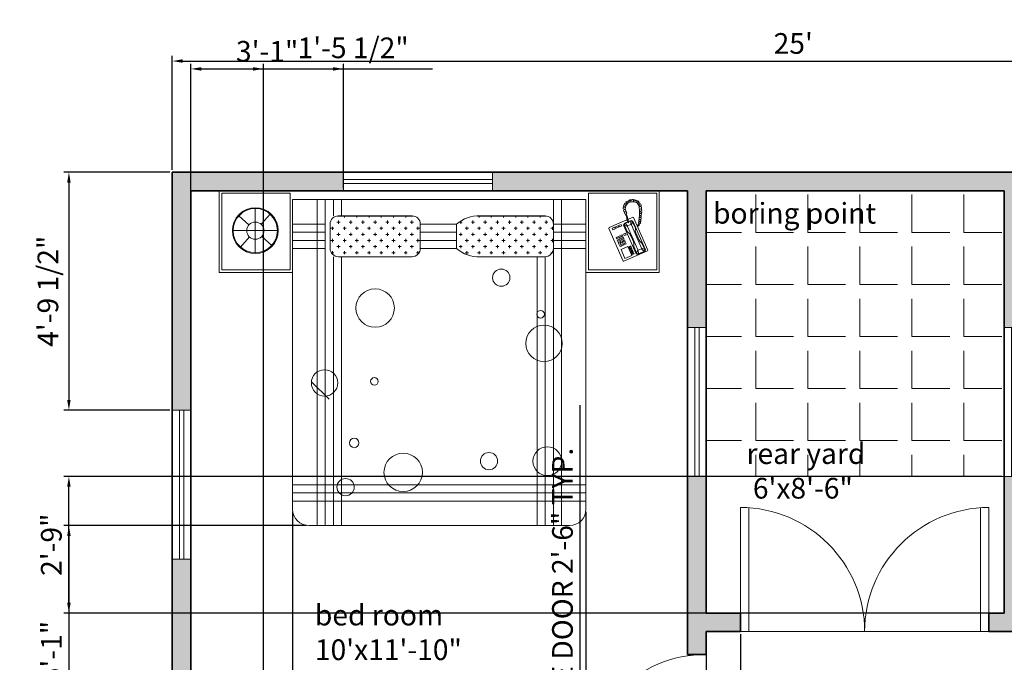
# Model space of a CAD drawing. Units: inches. Extents: x 2576 to 2974, y 2059 to 2656.
# Tile 3 of 4: x 2576 to 2814, y 2448 to 2604. Entities that reach past the tile are written whole.
import ezdxf

# ---------------------------------------------------------------- set-up
doc = ezdxf.new("R2010")
doc.units = ezdxf.units.IN
for name, color, linetype, lineweight in [('A-ANNO-DIMS', 101, 'Continuous', 18), ('A-ANNO-TEXT', 101, 'Continuous', 18), ('A-AREA-IDEN', 101, 'Continuous', 18), ('A-FLOR', 143, 'Continuous', 18), ('A-FLOR-PATT', 195, 'Continuous', 13), ('A-FURN-PATT', 195, 'Continuous', 13), ('A-WALL-PATT', 233, 'Continuous', 13), ('doors', 235, 'Continuous', 18), ('Furniture', 195, 'Continuous', 15), ('wall', 143, 'Continuous', 35), ('windows', 85, 'Continuous', 18)]:
    doc.layers.add(name, color=color, linetype=linetype, lineweight=lineweight)
doc.styles.get("Standard").update_dxf_attribs({"font": 'txt', "height": 5})
doc.dimstyles.new('ISO-25', dxfattribs={"dimtxt": 5, "dimasz": 2.5, "dimexe": 1.25, "dimexo": 0.625, "dimtad": 1, "dimlunit": 3, "dimtxsty": 'Standard', "dimcen": 2.5, "dimadec": 0, "dimazin": 0, "dimtfac": 1, "dimtmove": 0, "dimatfit": 3, "dimfxl": 1, "dimarcsym": 0})

# ---------------------------------------------------------------- blocks, each defined once
blk = doc.blocks.new('*D2')
at = {"layer": 'A-ANNO-DIMS', "color": 0, "lineweight": -2, "transparency": 16777216}
for p, q in [((2612.56, 2567.5), (2612.56, 2595)), ((2615.06, 2593.75), (2910.06, 2593.75)), ((2912.56, 2567.5), (2912.56, 2595))]:
    blk.add_line(p, q, dxfattribs=at)
at = {"layer": 'A-ANNO-DIMS', "color": 0, "transparency": 16777216}
for points in [[(2615.06, 2594.17), (2615.06, 2593.33), (2612.56, 2593.75)], [(2910.06, 2594.17), (2910.06, 2593.33), (2912.56, 2593.75)]]:
    blk.add_solid(points, dxfattribs=at)
at = {"layer": 'Defpoints', "color": 0, "transparency": 16777216}
for p in [(2912.56, 2593.75), (2612.56, 2566.88), (2912.56, 2566.88)]:
    blk.add_point(p, dxfattribs=at)
at = {"layer": 'A-ANNO-DIMS', "color": 0, "transparency": 16777216, "insert": (2762.56, 2597.35), "char_height": 5, "attachment_point": 5}
blk.add_mtext("25'", dxfattribs=at)
blk = doc.blocks.new('DOOR-SWING-30IN')
for p, q in [((0, 30), (30, 30)), ((30, 30), (30, 0)), ((0.07, 28), (30, 28))]:
    blk.add_line(p, q)
blk.add_arc((30, 30), 30, 180, 270)
blk = doc.blocks.new('DOOR-PAIR-60IN')
for p, q in [((0, 30), (0, 0)), ((2, 29.93), (2, 0)), ((58, 29.93), (58, 0)), ((60, 30), (60, 0)), ((0, 0), (30, 0)), ((60, 0), (30, 0))]:
    blk.add_line(p, q)
for centre, start, end in [((0, 0), 0, 90), ((60, 0), 90, 180)]:
    blk.add_arc(centre, 30, start, end)
blk = doc.blocks.new('WINDOW-36IN')
for p, q in [((0, 36), (0, 0)), ((4.5, 36), (0, 36)), ((1.75, 36), (1.75, 0)), ((2.75, 36), (2.75, 0)), ((4.5, 0), (4.5, 36)), ((0, 0), (4.5, 0))]:
    blk.add_line(p, q)
blk = doc.blocks.new('*D13')
at = {"layer": 'A-ANNO-DIMS', "color": 0, "lineweight": -2, "transparency": 16777216}
for p, q in [((2711.06, 2411.38), (2711.06, 2510.6)), ((2707.18, 2411.38), (2712.31, 2411.38)), ((2711.06, 2383.88), (2711.06, 2408.88)), ((2707.18, 2381.38), (2712.31, 2381.38))]:
    blk.add_line(p, q, dxfattribs=at)
at = {"layer": 'A-ANNO-DIMS', "color": 0, "transparency": 16777216}
for points in [[(2710.64, 2408.88), (2711.47, 2408.88), (2711.06, 2411.38)], [(2710.64, 2383.88), (2711.47, 2383.88), (2711.06, 2381.38)]]:
    blk.add_solid(points, dxfattribs=at)
at = {"layer": 'Defpoints', "color": 0, "transparency": 16777216}
for p in [(2706.56, 2411.38), (2711.06, 2411.38), (2706.56, 2381.38)]:
    blk.add_point(p, dxfattribs=at)
at = {"layer": 'A-ANNO-DIMS', "color": 0, "transparency": 16777216, "insert": (2707.46, 2462.24), "char_height": 5, "attachment_point": 5, "rotation": 90}
blk.add_mtext('SINGLE DOOR 2\'-6" TYP.', dxfattribs=at)
blk = doc.blocks.new('*D25')
at = {"layer": 'A-ANNO-DIMS', "color": 0, "lineweight": -2, "transparency": 16777216}
for p, q in [((2617.06, 2563), (2617.06, 2593.1)), ((2653.89, 2563), (2653.89, 2593.1)), ((2619.56, 2591.85), (2651.39, 2591.85))]:
    blk.add_line(p, q, dxfattribs=at)
at = {"layer": 'A-ANNO-DIMS', "color": 0, "transparency": 16777216}
for points in [[(2619.56, 2592.27), (2619.56, 2591.43), (2617.06, 2591.85)], [(2651.39, 2592.27), (2651.39, 2591.43), (2653.89, 2591.85)]]:
    blk.add_solid(points, dxfattribs=at)
at = {"layer": 'Defpoints', "color": 0, "transparency": 16777216}
for p in [(2653.89, 2591.85), (2617.06, 2562.38), (2653.89, 2562.38)]:
    blk.add_point(p, dxfattribs=at)
at = {"layer": 'A-ANNO-DIMS', "color": 0, "transparency": 16777216, "insert": (2635.47, 2595.45), "char_height": 5, "attachment_point": 5}
blk.add_mtext('3\'-1"', dxfattribs=at)
blk = doc.blocks.new('*D27')
at = {"layer": 'A-ANNO-DIMS', "color": 0, "lineweight": -2, "transparency": 16777216}
for p, q in [((2611.93, 2566.88), (2586.33, 2566.88)), ((2587.58, 2564.38), (2587.58, 2511.88)), ((2611.93, 2509.38), (2586.33, 2509.38))]:
    blk.add_line(p, q, dxfattribs=at)
at = {"layer": 'A-ANNO-DIMS', "color": 0, "transparency": 16777216}
for points in [[(2587.16, 2564.38), (2588, 2564.38), (2587.58, 2566.88)], [(2587.16, 2511.88), (2588, 2511.88), (2587.58, 2509.38)]]:
    blk.add_solid(points, dxfattribs=at)
at = {"layer": 'Defpoints', "color": 0, "transparency": 16777216}
for p in [(2612.56, 2566.88), (2587.58, 2509.38), (2612.56, 2509.38)]:
    blk.add_point(p, dxfattribs=at)
at = {"layer": 'A-ANNO-DIMS', "color": 0, "transparency": 16777216, "insert": (2583.15, 2538.13), "char_height": 5, "attachment_point": 5, "rotation": 90}
blk.add_mtext('4\'-9 1/2"', dxfattribs=at)
blk = doc.blocks.new('*D33')
at = {"layer": 'A-ANNO-DIMS', "color": 0, "lineweight": -2, "transparency": 16777216}
for p, q in [((2812.93, 2493.38), (2586.33, 2493.38)), ((2587.58, 2462.88), (2587.58, 2490.88)), ((2812.93, 2460.38), (2586.33, 2460.38))]:
    blk.add_line(p, q, dxfattribs=at)
at = {"layer": 'A-ANNO-DIMS', "color": 0, "transparency": 16777216}
for points in [[(2587.16, 2490.88), (2588, 2490.88), (2587.58, 2493.38)], [(2587.16, 2462.88), (2588, 2462.88), (2587.58, 2460.38)]]:
    blk.add_solid(points, dxfattribs=at)
at = {"layer": 'Defpoints', "color": 0, "transparency": 16777216}
for p in [(2587.58, 2493.38), (2813.56, 2493.38), (2813.56, 2460.38)]:
    blk.add_point(p, dxfattribs=at)
at = {"layer": 'A-ANNO-DIMS', "color": 0, "transparency": 16777216, "insert": (2583.98, 2476.88), "char_height": 5, "attachment_point": 5, "rotation": 90}
blk.add_mtext('2\'-9"', dxfattribs=at)
blk = doc.blocks.new('*D34')
at = {"layer": 'A-ANNO-DIMS', "color": 0, "lineweight": -2, "transparency": 16777216}
for p, q in [((2741.56, 2455.25), (2741.56, 2060.65)), ((2749.82, 2455.25), (2749.82, 2060.65)), ((2744.06, 2061.9), (2747.32, 2061.9)), ((2749.82, 2061.9), (2791.66, 2061.9))]:
    blk.add_line(p, q, dxfattribs=at)
at = {"layer": 'A-ANNO-DIMS', "color": 0, "transparency": 16777216}
for points in [[(2744.06, 2062.32), (2744.06, 2061.48), (2741.56, 2061.9)], [(2747.32, 2062.32), (2747.32, 2061.48), (2749.82, 2061.9)]]:
    blk.add_solid(points, dxfattribs=at)
at = {"layer": 'Defpoints', "color": 0, "transparency": 16777216}
for p in [(2741.56, 2455.88), (2749.82, 2455.88), (2749.82, 2061.9)]:
    blk.add_point(p, dxfattribs=at)
at = {"layer": 'A-ANNO-DIMS', "color": 0, "transparency": 16777216, "insert": (2771.99, 2066.34), "char_height": 5, "attachment_point": 5}
blk.add_mtext('0\'-8 1/2"', dxfattribs=at)
blk = doc.blocks.new('*D35')
at = {"layer": 'A-ANNO-DIMS', "color": 0, "lineweight": -2, "transparency": 16777216}
for p, q in [((2617.06, 2207), (2617.06, 2593.1)), ((2634.56, 2207), (2634.56, 2593.1)), ((2619.56, 2591.85), (2632.06, 2591.85)), ((2634.56, 2591.85), (2675.45, 2591.85))]:
    blk.add_line(p, q, dxfattribs=at)
at = {"layer": 'A-ANNO-DIMS', "color": 0, "transparency": 16777216}
for points in [[(2619.56, 2592.27), (2619.56, 2591.43), (2617.06, 2591.85)], [(2632.06, 2592.27), (2632.06, 2591.43), (2634.56, 2591.85)]]:
    blk.add_solid(points, dxfattribs=at)
at = {"layer": 'Defpoints', "color": 0, "transparency": 16777216}
for p in [(2634.56, 2591.85), (2617.06, 2206.38), (2634.56, 2206.38)]:
    blk.add_point(p, dxfattribs=at)
at = {"layer": 'A-ANNO-DIMS', "color": 0, "transparency": 16777216, "insert": (2656.25, 2596.29), "char_height": 5, "attachment_point": 5}
blk.add_mtext('1\'-5 1/2"', dxfattribs=at)
blk = doc.blocks.new('*D39')
at = {"layer": 'A-ANNO-DIMS', "color": 0, "lineweight": -2, "transparency": 16777216}
for p, q in [((2641.62, 2484.83), (2641.62, 2060.65)), ((2712.49, 2484.83), (2712.49, 2060.65)), ((2644.12, 2061.9), (2709.99, 2061.9))]:
    blk.add_line(p, q, dxfattribs=at)
at = {"layer": 'A-ANNO-DIMS', "color": 0, "transparency": 16777216}
for points in [[(2644.12, 2062.32), (2644.12, 2061.48), (2641.62, 2061.9)], [(2709.99, 2062.32), (2709.99, 2061.48), (2712.49, 2061.9)]]:
    blk.add_solid(points, dxfattribs=at)
at = {"layer": 'Defpoints', "color": 0, "transparency": 16777216}
for p in [(2641.62, 2485.45), (2712.49, 2485.45), (2712.49, 2061.9)]:
    blk.add_point(p, dxfattribs=at)
at = {"layer": 'A-ANNO-DIMS', "color": 0, "transparency": 16777216, "insert": (2677.06, 2065.5), "char_height": 5, "attachment_point": 5}
blk.add_mtext('5\'-11"', dxfattribs=at)
blk = doc.blocks.new('*D40')
at = {"layer": 'A-ANNO-DIMS', "color": 0, "lineweight": -2, "transparency": 16777216}
for p, q in [((2644.94, 2481.52), (2586.33, 2481.52)), ((2587.58, 2479.02), (2587.58, 2422.88)), ((2616.43, 2420.38), (2586.33, 2420.38))]:
    blk.add_line(p, q, dxfattribs=at)
at = {"layer": 'A-ANNO-DIMS', "color": 0, "transparency": 16777216}
for points in [[(2587.16, 2479.02), (2588, 2479.02), (2587.58, 2481.52)], [(2587.16, 2422.88), (2588, 2422.88), (2587.58, 2420.38)]]:
    blk.add_solid(points, dxfattribs=at)
at = {"layer": 'Defpoints', "color": 0, "transparency": 16777216}
for p in [(2645.56, 2481.52), (2587.58, 2420.38), (2617.06, 2420.38)]:
    blk.add_point(p, dxfattribs=at)
at = {"layer": 'A-ANNO-DIMS', "color": 0, "transparency": 16777216, "insert": (2583.98, 2450.95), "char_height": 5, "attachment_point": 5, "rotation": 90}
blk.add_mtext('5\'-1"', dxfattribs=at)

msp = doc.modelspace()

# ---------------------------------------------------------------- hatches: boundary and pattern name
at = {"layer": 'A-FLOR-PATT'}
h = msp.add_hatch(dxfattribs=at)
h.set_pattern_fill('ANGLE', color=256, scale=1.8)
h.set_pattern_definition([(0, (0, 0), (0, 12.573), [9.144, -3.429]), (90, (0, 0), (-12.573, 8e-16), [9.144, -3.429])])
h.paths.add_polyline_path([(2813.556, 2562.376), (2741.556, 2562.376), (2741.556, 2493.376), (2813.556, 2493.376), (2813.556, 2529.376)])
h.paths.add_polyline_path([(2750.035, 2495.142), (2809.21, 2495.142), (2809.21, 2502.647), (2750.035, 2502.647)], flags=24)
h.paths.add_polyline_path([(2741.924, 2553.087), (2815.278, 2553.087), (2815.278, 2560.74), (2741.924, 2560.74)], flags=9)
at = {"layer": 'A-FURN-PATT'}
h = msp.add_hatch(dxfattribs=at)
h.set_pattern_fill('CROSS', color=256, scale=5.9055, angle=360, style=0)
h.set_pattern_definition([(360, (2005.6814, 3287.0948), (1.476375, -1.476375), [0.7381875, -2.2145625]), (270, (2006.0505, 3287.464), (-1.476375, -1.476375), [0.7381875, -2.2145625])])
h.paths.add_polyline_path([(2672.476, 2548.447), (2672.476, 2554.352, 0.4142136), (2670.508, 2556.321), (2652.647, 2556.321, 0.4142136), (2650.678, 2554.352), (2650.678, 2548.447, 0.4142136), (2652.647, 2546.478), (2670.508, 2546.478, 0.4142136)])
h.paths.add_polyline_path([(2686.899, 2556.321, 0.1922305), (2681.232, 2554.352), (2681.232, 2548.447, 0.1922305), (2686.899, 2546.478), (2702.647, 2546.478, 0.4142136), (2704.615, 2548.447), (2704.615, 2554.352, 0.4142136), (2702.647, 2556.321)])
at = {"layer": 'A-WALL-PATT'}
h = msp.add_hatch(color=256, dxfattribs=at)
h.dxf.hatch_style = 1
h.paths.add_polyline_path([(2726.595, 2349.876), (2706.556, 2349.876), (2706.556, 2381.376), (2702.056, 2381.376), (2702.056, 2349.876), (2617.056, 2349.876), (2617.056, 2370.876), (2612.556, 2370.876), (2612.556, 2287.457), (2617.056, 2287.457), (2617.056, 2345.376), (2726.595, 2345.376)])
h.paths.add_polyline_path([(2823.556, 2345.376), (2828.056, 2345.376), (2828.056, 2349.876), (2808.018, 2349.876), (2808.018, 2345.376), (2819.056, 2345.376), (2819.056, 2206.376), (2748.056, 2206.376), (2748.056, 2201.876), (2819.056, 2201.876), (2819.056, 2159.528), (2823.556, 2159.528)])
h.paths.add_polyline_path([(2634.556, 2206.376), (2617.056, 2206.376), (2617.056, 2239.457), (2612.556, 2239.457), (2612.556, 2086.876), (2696.755, 2086.876), (2696.755, 2091.376), (2617.056, 2091.376), (2617.056, 2201.876), (2634.556, 2201.876)])
h.paths.add_polyline_path([(2688.056, 2206.376), (2670.556, 2206.376), (2670.556, 2201.876), (2688.056, 2201.876)], flags=17)
h.paths.add_polyline_path([(2832.708, 2091.376), (2732.755, 2091.376), (2732.755, 2086.876), (2832.708, 2086.876)])
h.paths.add_polyline_path([(2823.556, 2159.528), (2819.056, 2159.528), (2819.056, 2128.522), (2823.556, 2124.554)])
h.paths.add_polyline_path([(2840.936, 2566.876), (2689.889, 2566.876), (2689.889, 2562.376), (2730.206, 2562.376), (2737.056, 2562.376), (2737.056, 2529.376), (2741.556, 2529.376), (2741.556, 2562.376), (2813.556, 2562.376), (2813.556, 2529.376), (2818.056, 2529.376), (2818.056, 2562.376), (2840.936, 2562.376)])
h.paths.add_polyline_path([(2653.889, 2566.876), (2612.556, 2566.876), (2612.556, 2509.376), (2617.056, 2509.376), (2617.056, 2562.376), (2653.889, 2562.376)])
h.paths.add_polyline_path([(2822.556, 2460.376), (2818.056, 2460.376), (2818.056, 2493.376), (2813.556, 2493.376), (2813.556, 2460.376), (2809.817, 2460.376), (2809.817, 2455.876), (2822.556, 2455.876)])
h.paths.add_polyline_path([(2912.556, 2489.593), (2908.056, 2489.593), (2908.056, 2470.164), (2908.056, 2460.376), (2852.556, 2460.376), (2852.556, 2455.876), (2908.056, 2455.876), (2908.056, 2349.876), (2858.056, 2349.876), (2858.056, 2345.376), (2908.056, 2345.376), (2908.056, 2285.493), (2912.556, 2285.493)])
h.paths.add_polyline_path([(2749.817, 2460.376), (2741.556, 2460.376), (2741.556, 2493.376), (2737.056, 2493.376), (2737.056, 2450.376), (2741.556, 2450.376), (2741.556, 2455.876), (2749.817, 2455.876)])
h.paths.add_polyline_path([(2741.556, 2420.376), (2711.556, 2420.376), (2617.056, 2420.376), (2617.056, 2473.376), (2612.556, 2473.376), (2612.556, 2394.876), (2617.056, 2394.876), (2617.056, 2415.876), (2702.056, 2415.876), (2702.056, 2411.376), (2706.556, 2411.376), (2706.556, 2415.876), (2741.556, 2415.876)])
h.paths.add_polyline_path([(2912.556, 2566.876), (2876.936, 2566.876), (2876.936, 2562.376), (2908.056, 2562.376), (2908.056, 2525.593), (2912.556, 2525.593)])
h.paths.add_polyline_path([(2741.924, 2553.087), (2815.278, 2553.087), (2815.278, 2560.74), (2741.924, 2560.74)], flags=25)

# ---------------------------------------------------------------- linework, layer by layer
at = {"layer": 'A-FLOR'}
msp.add_line((2813.556, 2493.376), (2741.556, 2493.376), dxfattribs=at)
at = {"layer": 'Furniture'}
for p, q in [((2623.907, 2562.376), (2730.206, 2562.376)), ((2623.907, 2542.691), (2623.907, 2562.376)), ((2730.206, 2542.691), (2730.206, 2562.376)), ((2624.497, 2543.281), (2624.497, 2561.785)), ((2624.497, 2561.785), (2641.033, 2561.785)), ((2641.033, 2543.281), (2641.033, 2561.785)), ((2641.623, 2560.258), (2712.489, 2560.258)), ((2641.623, 2485.455), (2641.623, 2560.258)), ((2712.489, 2560.258), (2712.489, 2485.455)), ((2713.08, 2543.281), (2713.08, 2561.785)), ((2713.08, 2561.785), (2713.08, 2543.281)), ((2729.615, 2561.785), (2713.08, 2561.785)), ((2722.163, 2559.671), (2722.376, 2559.847)), ((2722.365, 2559.303), (2722.163, 2559.671)), ((2722.376, 2559.847), (2722.663, 2559.599)), ((2723.3, 2559.753), (2722.63, 2559.391)), ((2722.663, 2559.599), (2722.665, 2559.973)), ((2722.665, 2559.973), (2722.852, 2560.082)), ((2722.852, 2560.082), (2723.08, 2559.782)), ((2723.046, 2560.208), (2723.291, 2560.247)), ((2723.08, 2559.782), (2723.046, 2560.208)), ((2723.291, 2560.247), (2723.44, 2559.939)), ((2724.099, 2559.757), (2723.3, 2559.753)), ((2723.44, 2559.939), (2723.605, 2560.287)), ((2723.605, 2560.287), (2723.831, 2560.275)), ((2723.831, 2560.275), (2723.948, 2559.912)), ((2723.948, 2559.912), (2724.06, 2560.32)), ((2724.06, 2560.32), (2724.316, 2560.239)), ((2724.827, 2559.481), (2724.099, 2559.757)), ((2724.316, 2560.239), (2724.314, 2559.865)), ((2724.314, 2559.865), (2724.577, 2560.146)), ((2724.577, 2560.146), (2724.789, 2560.072)), ((2724.789, 2560.072), (2724.764, 2559.688)), ((2724.764, 2559.688), (2725.054, 2559.94)), ((2725.369, 2558.682), (2724.827, 2559.481)), ((2725.054, 2559.94), (2725.248, 2559.748)), ((2725.248, 2559.748), (2725.107, 2559.314)), ((2725.107, 2559.314), (2725.461, 2559.482)), ((2725.461, 2559.482), (2725.609, 2559.271)), ((2729.615, 2543.281), (2729.615, 2561.785)), ((2632.615, 2552.77), (2632.615, 2558.115)), ((2721.465, 2558.012), (2721.5, 2558.345)), ((2721.901, 2557.899), (2721.465, 2558.012)), ((2721.5, 2558.345), (2721.878, 2558.427)), ((2721.546, 2557.702), (2721.901, 2557.899)), ((2721.659, 2557.379), (2721.546, 2557.702)), ((2721.573, 2558.681), (2721.656, 2558.966)), ((2721.878, 2558.427), (2721.573, 2558.681)), ((2721.656, 2558.966), (2722.009, 2558.885)), ((2722.07, 2557.324), (2721.659, 2557.379)), ((2721.759, 2557.119), (2722.07, 2557.324)), ((2721.904, 2556.851), (2721.759, 2557.119)), ((2721.826, 2559.178), (2721.985, 2559.413)), ((2722.009, 2558.885), (2721.826, 2559.178)), ((2722.157, 2558.798), (2721.96, 2558.049)), ((2721.96, 2558.049), (2722.221, 2557.293)), ((2721.985, 2559.413), (2722.365, 2559.303)), ((2722.63, 2559.391), (2722.157, 2558.798)), ((2722.221, 2557.293), (2722.384, 2557.047)), ((2725.463, 2557.425), (2725.369, 2558.682)), ((2725.609, 2559.271), (2725.383, 2558.965)), ((2725.383, 2558.965), (2725.788, 2559.017)), ((2725.386, 2556.59), (2725.463, 2557.425)), ((2725.857, 2558.702), (2725.544, 2558.565)), ((2725.544, 2558.565), (2725.889, 2558.44)), ((2725.924, 2558.138), (2725.548, 2557.987)), ((2725.548, 2557.987), (2725.94, 2558.007)), ((2725.988, 2557.613), (2725.625, 2557.496)), ((2725.625, 2557.496), (2725.981, 2557.251)), ((2725.788, 2559.017), (2725.857, 2558.702)), ((2725.889, 2558.44), (2725.924, 2558.138)), ((2725.981, 2557.251), (2725.934, 2557.009)), ((2725.94, 2558.007), (2725.988, 2557.613)), ((2631.083, 2554.16), (2628.656, 2556.36)), ((2634.005, 2554.303), (2636.205, 2556.729)), ((2670.743, 2556.307), (2652.412, 2556.307)), ((2668.479, 2556.307), (2668.465, 2556.321)), ((2702.882, 2556.307), (2686.664, 2556.307)), ((2722.402, 2555.365), (2718.109, 2553.489)), ((2722.551, 2554.884), (2721.746, 2554.532)), ((2722.087, 2556.779), (2721.904, 2556.851)), ((2721.943, 2554.55), (2722.575, 2554.827)), ((2722.083, 2556.694), (2722.087, 2556.779)), ((2722.226, 2556.397), (2722.083, 2556.694)), ((2722.325, 2555.792), (2722.226, 2556.397)), ((2722.384, 2557.047), (2722.242, 2556.805)), ((2722.242, 2556.805), (2722.385, 2556.508)), ((2722.44, 2555.151), (2722.325, 2555.792)), ((2722.385, 2556.508), (2722.472, 2556.215)), ((2722.648, 2554.654), (2722.44, 2555.151)), ((2722.472, 2556.215), (2722.571, 2555.609)), ((2722.571, 2555.609), (2722.652, 2555.202)), ((2723.836, 2555.992), (2722.602, 2555.452)), ((2722.819, 2554.729), (2722.648, 2554.654)), ((2722.652, 2555.202), (2722.819, 2554.729)), ((2723.407, 2555.258), (2722.736, 2554.965)), ((2722.757, 2554.906), (2723.317, 2555.151)), ((2723.317, 2555.151), (2723.596, 2555.136)), ((2723.356, 2554.281), (2723.317, 2555.151)), ((2723.843, 2555.04), (2723.407, 2555.258)), ((2723.754, 2554.932), (2723.463, 2554.192)), ((2723.596, 2555.136), (2723.754, 2554.932)), ((2723.754, 2554.932), (2724.429, 2553.386)), ((2724.001, 2555.927), (2723.836, 2555.992)), ((2726.846, 2548.167), (2723.843, 2555.04)), ((2727.455, 2548.024), (2724.001, 2555.927)), ((2725.201, 2554.645), (2725.257, 2555.084)), ((2725.257, 2555.084), (2725.355, 2555.872)), ((2725.355, 2555.872), (2725.39, 2556.454)), ((2725.461, 2556.513), (2725.386, 2556.59)), ((2725.73, 2555.014), (2725.388, 2554.975)), ((2725.388, 2554.975), (2725.705, 2554.755)), ((2725.39, 2556.454), (2725.461, 2556.513)), ((2725.796, 2555.526), (2725.414, 2555.484)), ((2725.414, 2555.484), (2725.746, 2555.228)), ((2725.821, 2555.91), (2725.447, 2555.913)), ((2725.447, 2555.913), (2725.807, 2555.752)), ((2725.859, 2556.424), (2725.5, 2556.392)), ((2725.5, 2556.392), (2725.825, 2556.216)), ((2725.934, 2557.009), (2725.569, 2556.96)), ((2725.569, 2556.96), (2725.88, 2556.723)), ((2725.705, 2554.755), (2725.714, 2554.607)), ((2725.746, 2555.228), (2725.73, 2555.014)), ((2725.807, 2555.752), (2725.796, 2555.526)), ((2725.825, 2556.216), (2725.821, 2555.91)), ((2725.88, 2556.723), (2725.859, 2556.424)), ((2632.615, 2552.77), (2627.271, 2552.77)), ((2632.615, 2552.77), (2632.615, 2547.426)), ((2632.615, 2552.77), (2637.96, 2552.77)), ((2718.109, 2553.489), (2718.045, 2553.324)), ((2718.045, 2553.324), (2721.498, 2545.421)), ((2718.857, 2553.338), (2719.43, 2553.588)), ((2719.007, 2552.995), (2718.857, 2553.338)), ((2719.58, 2553.245), (2719.007, 2552.995)), ((2719.43, 2553.588), (2719.58, 2553.245)), ((2719.659, 2553.689), (2720.232, 2553.939)), ((2719.809, 2553.345), (2719.659, 2553.689)), ((2720.382, 2553.595), (2719.809, 2553.345)), ((2720.232, 2553.939), (2720.382, 2553.595)), ((2720.461, 2554.039), (2721.033, 2554.289)), ((2720.611, 2553.695), (2720.461, 2554.039)), ((2721.184, 2553.946), (2720.611, 2553.695)), ((2721.033, 2554.289), (2721.184, 2553.946)), ((2721.746, 2554.532), (2721.584, 2554.121)), ((2721.584, 2554.121), (2724.613, 2547.191)), ((2721.943, 2554.55), (2721.763, 2554.335)), ((2721.763, 2554.335), (2721.806, 2554.081)), ((2721.806, 2554.081), (2722.482, 2552.535)), ((2721.806, 2554.081), (2722.547, 2553.791)), ((2722.554, 2553.931), (2721.943, 2554.55)), ((2722.482, 2552.535), (2722.722, 2552.299)), ((2722.547, 2553.791), (2722.554, 2553.931)), ((2723.898, 2550.699), (2722.547, 2553.791)), ((2723.356, 2554.281), (2722.554, 2553.931)), ((2722.722, 2552.299), (2723.019, 2552.087)), ((2723.463, 2554.192), (2723.356, 2554.281)), ((2724.815, 2551.099), (2723.463, 2554.192)), ((2724.44, 2553.05), (2724.393, 2552.688)), ((2724.393, 2552.688), (2724.511, 2552.262)), ((2724.429, 2553.386), (2724.44, 2553.05)), ((2724.852, 2553.98), (2725.043, 2554.12)), ((2725.229, 2553.98), (2724.927, 2553.808)), ((2725.043, 2554.12), (2725.13, 2554.269)), ((2725.13, 2554.269), (2725.235, 2554.439)), ((2725.39, 2554.59), (2725.201, 2554.645)), ((2725.332, 2554.122), (2725.229, 2553.98)), ((2725.235, 2554.439), (2725.275, 2554.539)), ((2725.275, 2554.539), (2725.39, 2554.59)), ((2725.398, 2554.414), (2725.332, 2554.122)), ((2725.602, 2554.516), (2725.398, 2554.414)), ((2725.714, 2554.607), (2725.602, 2554.516)), ((2631.226, 2551.238), (2629.026, 2548.811)), ((2634.148, 2551.381), (2636.574, 2549.181)), ((2720.094, 2551.287), (2719.751, 2551.137)), ((2719.751, 2551.137), (2719.901, 2550.793)), ((2719.901, 2550.793), (2720.245, 2550.943)), ((2720.37, 2550.657), (2720.026, 2550.507)), ((2720.026, 2550.507), (2720.176, 2550.163)), ((2720.245, 2550.943), (2720.094, 2551.287)), ((2720.176, 2550.163), (2720.52, 2550.313)), ((2720.645, 2550.027), (2720.301, 2549.877)), ((2720.667, 2551.537), (2720.324, 2551.387)), ((2720.324, 2551.387), (2720.474, 2551.044)), ((2720.52, 2550.313), (2720.37, 2550.657)), ((2720.474, 2551.044), (2720.817, 2551.194)), ((2720.942, 2550.907), (2720.599, 2550.757)), ((2720.599, 2550.757), (2720.749, 2550.414)), ((2720.795, 2549.684), (2720.645, 2550.027)), ((2720.817, 2551.194), (2720.667, 2551.537)), ((2720.749, 2550.414), (2721.093, 2550.564)), ((2721.218, 2550.277), (2720.874, 2550.127)), ((2720.874, 2550.127), (2721.024, 2549.784)), ((2721.24, 2551.788), (2720.896, 2551.637)), ((2720.896, 2551.637), (2721.046, 2551.294)), ((2721.093, 2550.564), (2720.942, 2550.907)), ((2721.024, 2549.784), (2721.368, 2549.934)), ((2721.046, 2551.294), (2721.39, 2551.444)), ((2721.515, 2551.158), (2721.172, 2551.007)), ((2721.172, 2551.007), (2721.322, 2550.664)), ((2721.368, 2549.934), (2721.218, 2550.277)), ((2721.39, 2551.444), (2721.24, 2551.788)), ((2721.322, 2550.664), (2721.665, 2550.814)), ((2721.79, 2550.528), (2721.447, 2550.378)), ((2721.447, 2550.378), (2721.597, 2550.034)), ((2721.665, 2550.814), (2721.515, 2551.158)), ((2722.042, 2552.138), (2721.584, 2551.938)), ((2721.584, 2551.938), (2721.734, 2551.594)), ((2721.597, 2550.034), (2721.941, 2550.184)), ((2721.734, 2551.594), (2722.192, 2551.794)), ((2721.941, 2550.184), (2721.79, 2550.528)), ((2722.192, 2551.794), (2722.042, 2552.138)), ((2723.019, 2552.087), (2723.251, 2551.712)), ((2723.251, 2551.712), (2723.727, 2550.623)), ((2723.977, 2550.051), (2723.727, 2550.623)), ((2723.898, 2550.699), (2725.025, 2548.121)), ((2724.095, 2549.625), (2723.977, 2550.051)), ((2724.511, 2552.262), (2724.987, 2551.174)), ((2724.815, 2551.099), (2725.941, 2548.522)), ((2725.237, 2550.601), (2724.987, 2551.174)), ((2725.469, 2550.225), (2725.237, 2550.601)), ((2725.766, 2550.014), (2725.469, 2550.225)), ((2726.006, 2549.778), (2725.766, 2550.014)), ((2720.301, 2549.877), (2720.452, 2549.533)), ((2720.452, 2549.533), (2720.795, 2549.684)), ((2720.92, 2549.397), (2720.577, 2549.247)), ((2720.577, 2549.247), (2720.727, 2548.903)), ((2720.727, 2548.903), (2721.071, 2549.054)), ((2721.071, 2549.054), (2720.92, 2549.397)), ((2722.631, 2548.917), (2720.97, 2548.191)), ((2720.97, 2548.191), (2721.896, 2546.072)), ((2721.493, 2549.647), (2721.149, 2549.497)), ((2721.149, 2549.497), (2721.3, 2549.154)), ((2721.3, 2549.154), (2721.643, 2549.304)), ((2721.643, 2549.304), (2721.493, 2549.647)), ((2721.663, 2545.356), (2727.39, 2547.859)), ((2722.066, 2549.898), (2721.722, 2549.748)), ((2721.722, 2549.748), (2721.872, 2549.404)), ((2721.872, 2549.404), (2722.216, 2549.554)), ((2722.216, 2549.554), (2722.066, 2549.898)), ((2723.557, 2546.798), (2722.631, 2548.917)), ((2722.853, 2548.877), (2723.311, 2549.078)), ((2722.928, 2548.706), (2722.853, 2548.877)), ((2723.386, 2548.906), (2722.928, 2548.706)), ((2723.003, 2548.534), (2723.461, 2548.734)), ((2723.078, 2548.362), (2723.003, 2548.534)), ((2723.536, 2548.562), (2723.078, 2548.362)), ((2723.153, 2548.19), (2723.611, 2548.39)), ((2723.228, 2548.018), (2723.153, 2548.19)), ((2723.686, 2548.219), (2723.228, 2548.018)), ((2723.303, 2547.847), (2723.761, 2548.047)), ((2723.378, 2547.675), (2723.303, 2547.847)), ((2723.311, 2549.078), (2723.386, 2548.906)), ((2723.836, 2547.875), (2723.378, 2547.675)), ((2723.453, 2547.503), (2723.911, 2547.703)), ((2723.461, 2548.734), (2723.536, 2548.562)), ((2723.611, 2548.39), (2723.686, 2548.219)), ((2723.761, 2548.047), (2723.836, 2547.875)), ((2723.911, 2547.703), (2723.987, 2547.531)), ((2724.048, 2549.263), (2724.095, 2549.625)), ((2724.059, 2548.927), (2724.048, 2549.263)), ((2724.734, 2547.381), (2724.059, 2548.927)), ((2724.734, 2547.381), (2725.025, 2548.121)), ((2724.967, 2547.005), (2726.685, 2547.756)), ((2725.025, 2548.121), (2725.132, 2548.032)), ((2725.934, 2548.382), (2725.132, 2548.032)), ((2725.132, 2548.032), (2725.171, 2547.162)), ((2725.171, 2547.162), (2726.545, 2547.763)), ((2725.941, 2548.522), (2725.934, 2548.382)), ((2725.934, 2548.382), (2726.545, 2547.763)), ((2726.682, 2548.232), (2725.941, 2548.522)), ((2726.682, 2548.232), (2726.006, 2549.778)), ((2726.545, 2547.763), (2726.724, 2547.977)), ((2726.724, 2547.977), (2726.682, 2548.232)), ((2726.685, 2547.756), (2726.846, 2548.167)), ((2727.39, 2547.859), (2727.455, 2548.024)), ((2721.498, 2545.421), (2721.663, 2545.356)), ((2721.896, 2546.072), (2723.557, 2546.798)), ((2723.528, 2547.331), (2723.453, 2547.503)), ((2723.987, 2547.531), (2723.528, 2547.331)), ((2723.603, 2547.159), (2724.062, 2547.36)), ((2723.679, 2546.987), (2723.603, 2547.159)), ((2724.137, 2547.188), (2723.679, 2546.987)), ((2724.062, 2547.36), (2724.137, 2547.188)), ((2724.613, 2547.191), (2724.967, 2547.005)), ((2724.892, 2547.177), (2724.734, 2547.381)), ((2725.171, 2547.162), (2724.892, 2547.177)), ((2624.497, 2543.281), (2641.033, 2543.281)), ((2729.615, 2543.281), (2713.08, 2543.281)), ((2623.907, 2542.691), (2641.623, 2542.691)), ((2730.206, 2542.691), (2712.489, 2542.691)), ((2650.421, 2512.015), (2646.163, 2516.273)), ((2706.584, 2507.034), (2706.523, 2507.094)), ((2708.552, 2481.518), (2645.56, 2481.518))]:
    msp.add_line(p, q, dxfattribs=at)
for points in [[(2649.497, 2560.258), (2649.497, 2481.518), (2647.529, 2481.518), (2647.529, 2560.258)], [(2651.466, 2556.321), (2651.466, 2560.258)], [(2653.434, 2560.258), (2653.434, 2556.321)], [(2704.615, 2560.258), (2704.615, 2481.518), (2706.584, 2481.518), (2706.584, 2560.258)], [(2649.497, 2554.352), (2641.623, 2554.352), (2641.623, 2552.384), (2649.497, 2552.384)], [(2681.232, 2554.352), (2672.476, 2554.352)], [(2672.476, 2552.384), (2681.232, 2552.384)], [(2712.489, 2554.352), (2704.615, 2554.352)], [(2704.615, 2552.384), (2712.489, 2552.384), (2712.489, 2554.352)], [(2649.497, 2550.415), (2641.623, 2550.415), (2641.623, 2548.447), (2649.497, 2548.447)], [(2681.232, 2550.415), (2672.476, 2550.415)], [(2704.615, 2548.447), (2712.489, 2548.447), (2712.489, 2550.415)], [(2712.489, 2550.415), (2704.615, 2550.415)], [(2672.476, 2548.447), (2681.232, 2548.447)], [(2653.434, 2546.478), (2653.434, 2481.518), (2651.466, 2481.518), (2651.466, 2546.478)], [(2700.678, 2546.478), (2700.678, 2481.518), (2702.647, 2481.518), (2702.647, 2546.478)]]:
    msp.add_lwpolyline(points, dxfattribs=at)
for points in [[(2652.647, 2546.478), (2670.508, 2546.478, 0.4142136), (2672.476, 2548.447), (2672.476, 2554.352, 0.4142136), (2670.508, 2556.321), (2652.647, 2556.321, 0.4142136), (2650.678, 2554.352), (2650.678, 2548.447, 0.4142136)], [(2686.899, 2546.478), (2702.647, 2546.478, 0.4142136), (2704.615, 2548.447), (2704.615, 2554.352, 0.4142136), (2702.647, 2556.321), (2686.899, 2556.321, 0.1922305), (2681.232, 2554.352), (2681.232, 2548.447, 0.1922305)]]:
    msp.add_lwpolyline(points, format="xyb", close=True, dxfattribs=at)
for points in [[(2712.489, 2493.329), (2641.623, 2493.329), (2641.623, 2491.36), (2712.489, 2491.36)], [(2712.489, 2489.392), (2641.623, 2489.392), (2641.623, 2487.423), (2712.489, 2487.423)]]:
    msp.add_lwpolyline(points, close=True, dxfattribs=at)
for centre, radius in [((2632.615, 2552.77), 5.541), ((2632.615, 2552.77), 5.344), ((2632.615, 2552.77), 2.069), ((2692.035, 2541.405), 2.087), ((2661.563, 2534.063), 4.646), ((2701.523, 2532.567), 0.925), ((2702.35, 2525.519), 4.409), ((2649.338, 2515.972), 3.189), ((2661.385, 2516.327), 0.925), ((2656.504, 2501.464), 1.142), ((2703.157, 2497.055), 3.484), ((2668.334, 2494.358), 4.646), ((2689.062, 2497.075), 2.087), ((2654.417, 2490.795), 2.087)]:
    msp.add_circle(centre, radius, dxfattribs=at)
for centre, start, end in [((2645.56, 2485.455), 180, 270), ((2708.552, 2485.455), 270, 0)]:
    msp.add_arc(centre, 3.937, start, end, dxfattribs=at)
at = {"layer": 'wall'}
for p, q in [((2612.556, 2566.876), (2912.556, 2566.876)), ((2612.556, 2086.876), (2612.556, 2566.876)), ((2617.056, 2562.376), (2737.056, 2562.376)), ((2617.056, 2420.376), (2617.056, 2562.376)), ((2737.056, 2450.376), (2737.056, 2562.376)), ((2741.556, 2562.376), (2813.556, 2562.376)), ((2741.556, 2460.376), (2741.556, 2562.376)), ((2813.556, 2460.376), (2813.556, 2562.376)), ((2741.556, 2460.376), (2749.817, 2460.376)), ((2749.817, 2460.376), (2749.817, 2455.876)), ((2809.817, 2460.376), (2809.817, 2455.876)), ((2809.817, 2460.376), (2813.556, 2460.376)), ((2741.556, 2455.876), (2749.817, 2455.876)), ((2741.556, 2450.376), (2741.556, 2455.876)), ((2809.817, 2455.876), (2822.556, 2455.876)), ((2737.056, 2450.376), (2741.556, 2450.376))]:
    msp.add_line(p, q, dxfattribs=at)

# ---------------------------------------------------------------- block references
at = {"layer": 'doors'}
msp.add_blockref('DOOR-PAIR-60IN', (2749.816, 2455.876), dxfattribs=at)
at = {"layer": 'doors', "extrusion": (0, 0, -1), "zscale": -1, "rotation": 180}
msp.add_blockref('DOOR-SWING-30IN', (-2711.556, 2450.376), dxfattribs=at)
at = {"layer": 'windows', "rotation": 89.99999999999731}
msp.add_blockref('WINDOW-36IN', (2689.888, 2562.376), dxfattribs=at)
at = {"layer": 'windows'}
for p in [(2737.056, 2493.376), (2813.556, 2493.376), (2612.556, 2473.376)]:
    msp.add_blockref('WINDOW-36IN', p, dxfattribs=at)

# ---------------------------------------------------------------- texts
at = {"layer": 'A-ANNO-TEXT'}
msp.add_text('boring point', height=5, dxfattribs=at).set_placement((2743.199, 2554.464))
at = {"layer": 'A-AREA-IDEN'}
for s, p in [('rear yard', (2751.286, 2496.397)), (' 6\'x8\'-6"', (2751.286, 2488.028)), ('bed room', (2647.008, 2457.378)), ('10\'x11\'-10"', (2647.008, 2449.009))]:
    msp.add_text(s, height=5, dxfattribs=at).set_placement(p)

# ---------------------------------------------------------------- dimensions: what is measured, and where the dimension line sits
at = {"layer": 'A-ANNO-DIMS'}
for base, p1, p2, override, picture, middle in [((2634.556, 2591.851), (2617.056, 2206.376), (2634.556, 2206.376), {"dimdec": 1, "dimlfac": 1, "dimrnd": 0, "dimzin": 1, "dimdsep": 46, "dimlunit": 4, "dimfrac": 2}, '*D35', (2656.253, 2596.285)), ((2912.556, 2593.75), (2612.556, 2566.876), (2912.556, 2566.876), {"dimclrd": 0, "dimclre": 0, "dimclrt": 0}, '*D2', (2762.556, 2597.351)), ((2653.889, 2591.851), (2617.056, 2562.376), (2653.889, 2562.376), {"dimdec": 1, "dimlfac": 1, "dimrnd": 0, "dimzin": 1, "dimdsep": 46, "dimlunit": 4, "dimfrac": 2}, '*D25', (2635.472, 2595.452)), ((2712.489, 2061.901), (2641.623, 2485.455), (2712.489, 2485.455), {"dimdec": 1, "dimlfac": 1, "dimrnd": 0, "dimzin": 1, "dimdsep": 46, "dimlunit": 4, "dimfrac": 2}, '*D39', (2677.056, 2065.502)), ((2749.817, 2061.901), (2741.556, 2455.876), (2749.817, 2455.876), {"dimdec": 1, "dimlfac": 1, "dimrnd": 0, "dimzin": 1, "dimdsep": 46, "dimlunit": 4, "dimfrac": 2}, '*D34', (2771.989, 2066.335))]:
    dim = msp.add_linear_dim(base=base, p1=p1, p2=p2, dimstyle='ISO-25', override=override, dxfattribs=at)
    dim.commit()
    dim.dimension.update_dxf_attribs({"geometry": picture, "text_midpoint": middle})
for base, p1, p2, picture, middle in [((2587.581, 2509.376), (2612.556, 2566.876), (2612.556, 2509.376), '*D27', (2583.147, 2538.126)), ((2587.581, 2493.376), (2813.556, 2460.376), (2813.556, 2493.376), '*D33', (2583.98, 2476.876)), ((2587.581, 2420.376), (2645.56, 2481.518), (2617.056, 2420.376), '*D40', (2583.98, 2450.947))]:
    dim = msp.add_linear_dim(base=base, p1=p1, p2=p2, angle=90, dimstyle='ISO-25', override={"dimdec": 1, "dimlfac": 1, "dimrnd": 0, "dimzin": 1, "dimdsep": 46, "dimlunit": 4, "dimfrac": 2}, dxfattribs=at)
    dim.commit()
    dim.dimension.update_dxf_attribs({"geometry": picture, "text_midpoint": middle})
dim = msp.add_linear_dim(base=(2711.056, 2411.376), p1=(2706.556, 2381.376), p2=(2706.556, 2411.376), angle=90, text='SINGLE DOOR <> TYP.', dimstyle='ISO-25', override={"dimdec": 1, "dimlfac": 1, "dimrnd": 0, "dimzin": 1, "dimdsep": 46, "dimlunit": 4, "dimfrac": 2}, dxfattribs=at)
dim.commit()
dim.dimension.update_dxf_attribs({"geometry": '*D13', "text_midpoint": (2707.455, 2462.239)})

doc.saveas('drawing.dxf')
